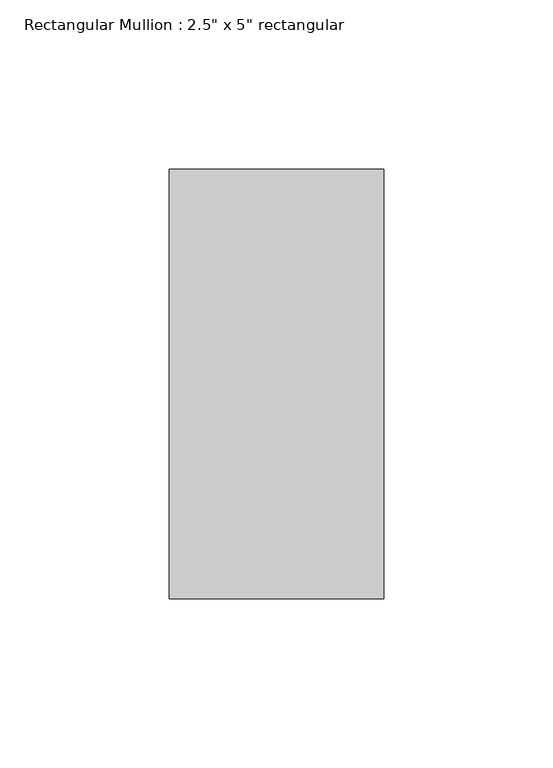
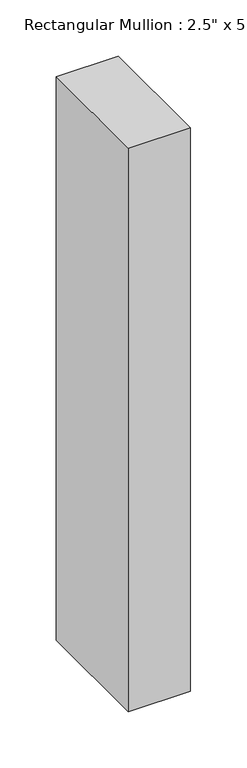
"""IFC4 building model written with IfcOpenShell, lengths in millimetres: member geometry."""

from ifc_helpers import new_model, si_unit, frame, origin, place, context, project, spatial, polyline, outline, extrude, source, transform, mapped, element, save


def member_47bfaf8a(model_context):
    return source(origin(), model_context, "Body", "SweptSolid", [
        extrude(outline(polyline([(0.0, 63.5), (0.0, -63.5), (-63.5, -63.5), (-63.5, 63.5), (0.0, 63.5)])), frame((0.0, 0.0, -609.6), z_axis=(0.0, 0.0, 1.0), x_axis=(1.0, 0.0, 0.0)), (0.0, 0.0, 1.0), 609.6),
    ])


if __name__ == "__main__":
    model = new_model("IFC4")
    model_context = context("Model", 3, world=origin())
    ifc_project = project(units=[si_unit("LENGTHUNIT", "METRE", prefix="MILLI")], contexts=[model_context])
    site = spatial("IfcSite", under=ifc_project)
    building = spatial("IfcBuilding", under=site)
    placement = place(None, origin())
    member_shape = member_47bfaf8a(model_context)
    element("IfcMember", 1, ObjectType="Rectangular Mullion : 2.5\" x 5\" rectangular", at=placement, inside=building, context=model_context, shape_type="MappedRepresentation", body=[
        mapped(member_shape, transform((0.0, 0.0, 0.0), x_axis=(1.0, 0.0, 0.0), y_axis=(0.0, 1.0, 0.0), z_axis=(0.0, 0.0, 1.0))),
    ])
    save(model, "model.ifc")

# Revit data of these elements
# Type "Rectangular Mullion : 2.5\" x 5\" rectangular"
#   built-in parameter 1007304 = 0.416667 (stored number, unit not read)
#   built-in parameter 1007301 = 0.104167 (stored number, unit not read)
#   built-in parameter 1007300 = 0.104167 (stored number, unit not read)
# Element 1 (IfcMember, "Rectangular Mullion : 2.5\" x 5\" rectangular")
#   Materials on its faces: "Aluminum"
# Materials
#   "Aluminum": class "Metal", colour RGB 247 247 247, transparency 0, Description = "Aluminum 6061", Cost = 0
